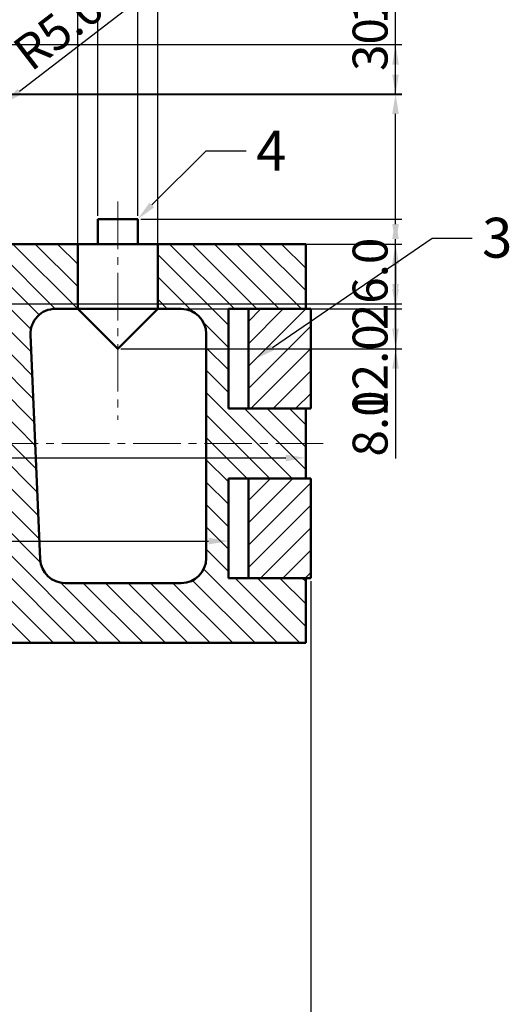
# Model space of a CAD drawing. Units: millimetres. Extents: x -21 to 693, y -570 to 295.
# Tile 5 of 7: x 253 to 352, y -4 to 193. Entities that reach past the tile are written whole.
import ezdxf
from ezdxf import colors
from ezdxf.entities.mleader import LeaderData, LeaderLine
from ezdxf.math import Vec2, Vec3

# ---------------------------------------------------------------- set-up
doc = ezdxf.new("R2010")
doc.units = ezdxf.units.MM
doc.header["$LTSCALE"] = 0.5
doc.linetypes.add('CENTER2', pattern=[28.575, 19.05, -3.175, 3.175, -3.175])
for name, color, linetype, lineweight in [('M-CNTR', 1, 'CENTER2', 18), ('M-DIMS', 2, 'Continuous', 25), ('M-HATC', 8, 'Continuous', 18), ('M-OUTL', 7, 'Continuous', 50), ('M-TEXT', 3, 'Continuous', 25)]:
    doc.layers.add(name, color=color, linetype=linetype, lineweight=lineweight)
doc.styles.get("Standard").update_dxf_attribs({"font": 'arial.ttf'})
doc.dimstyles.new('ISO-25', dxfattribs={"dimtxt": 7, "dimasz": 4, "dimexe": 1.25, "dimexo": 0.625, "dimtad": 1, "dimdec": 0, "dimtxsty": 'Standard', "dimcen": 2.5, "dimadec": 0, "dimazin": 0, "dimtfac": 1, "dimtdec": 0, "dimtofl": 0, "dimtmove": 0, "dimatfit": 3, "dimfxl": 1, "dimarcsym": 0})

# ---------------------------------------------------------------- blocks, each defined once
blk = doc.blocks.new('*U2')
at = {"layer": 'M-CNTR', "color": 0, "transparency": 16777216}
blk.add_line((90.5, 0), (-90.5, 0), dxfattribs=at)
blk = doc.blocks.new('*U4')
at = {"layer": 'M-CNTR', "color": 0, "transparency": 16777216}
blk.add_line((0, 6), (0, -37.73), dxfattribs=at)
blk = doc.blocks.new('*D5')
at = {"layer": 'Defpoints', "color": 0, "ltscale": 0.5, "transparency": 16777216}
for p in [(135.24, 81.11), (311.24, 81.11), (311.24, -8.97)]:
    blk.add_point(p, dxfattribs=at)
at = {"layer": 'M-DIMS', "color": 0, "lineweight": -2, "ltscale": 0.5, "transparency": 16777216}
for p, q in [((135.24, 80.49), (135.24, -10.22)), ((311.24, 80.49), (311.24, -10.22)), ((139.24, -8.97), (307.24, -8.97))]:
    blk.add_line(p, q, dxfattribs=at)
at = {"layer": 'M-DIMS', "color": 0, "ltscale": 0.5, "transparency": 16777216}
for points in [[(139.24, -8.31), (139.24, -9.64), (135.24, -8.97)], [(307.24, -8.31), (307.24, -9.64), (311.24, -8.97)]]:
    blk.add_solid(points, dxfattribs=at)
at = {"layer": 'M-DIMS', "color": 0, "ltscale": 0.5, "transparency": 16777216, "insert": (223.24, -4.58), "char_height": 7, "attachment_point": 5}
blk.add_mtext('%%C175', dxfattribs=at)
blk = doc.blocks.new('*D13')
at = {"layer": 'Defpoints', "color": 0, "ltscale": 0.5, "transparency": 16777216}
for p in [(151.74, 91.11), (294.74, 91.11), (294.74, 88.53)]:
    blk.add_point(p, dxfattribs=at)
at = {"layer": 'M-DIMS', "color": 0, "lineweight": -2, "ltscale": 0.5, "transparency": 16777216}
for p, q in [((151.74, 90.49), (151.74, 87.28)), ((294.74, 90.49), (294.74, 87.28)), ((155.74, 88.53), (290.74, 88.53))]:
    blk.add_line(p, q, dxfattribs=at)
at = {"layer": 'M-DIMS', "color": 0, "ltscale": 0.5, "transparency": 16777216}
for points in [[(155.74, 89.2), (155.74, 87.87), (151.74, 88.53)], [(290.74, 89.2), (290.74, 87.87), (294.74, 88.53)]]:
    blk.add_solid(points, dxfattribs=at)
at = {"layer": 'M-DIMS', "color": 0, "ltscale": 0.5, "transparency": 16777216, "insert": (223.24, 92.93), "char_height": 7, "attachment_point": 5}
blk.add_mtext('%%C158.5', dxfattribs=at)
blk = doc.blocks.new('*D14')
at = {"layer": 'Defpoints', "color": 0, "ltscale": 0.5, "transparency": 16777216}
for p in [(136.24, 108.11), (310.24, 108.11), (310.24, 105.22)]:
    blk.add_point(p, dxfattribs=at)
at = {"layer": 'M-DIMS', "color": 0, "lineweight": -2, "ltscale": 0.5, "transparency": 16777216}
for p, q in [((136.24, 107.49), (136.24, 103.97)), ((310.24, 107.49), (310.24, 103.97)), ((140.24, 105.22), (306.24, 105.22))]:
    blk.add_line(p, q, dxfattribs=at)
at = {"layer": 'M-DIMS', "color": 0, "ltscale": 0.5, "transparency": 16777216}
for points in [[(140.24, 105.89), (140.24, 104.55), (136.24, 105.22)], [(306.24, 105.89), (306.24, 104.55), (310.24, 105.22)]]:
    blk.add_solid(points, dxfattribs=at)
at = {"layer": 'M-DIMS', "color": 0, "ltscale": 0.5, "transparency": 16777216, "insert": (223.24, 109.62), "char_height": 7, "attachment_point": 5}
blk.add_mtext('%%C174', dxfattribs=at)
blk = doc.blocks.new('SCREW-PLUG')
for p, q in [((4, 21), (4, 26)), ((4, 26), (12, 26)), ((12, 26), (12, 21)), ((0, 21), (0, 8)), ((16, 21), (16, 8)), ((0, 8), (8, 0)), ((16, 8), (8, 0))]:
    blk.add_line(p, q)
blk = doc.blocks.new('*D55')
at = {"layer": 'Defpoints', "color": 0, "ltscale": 0.5, "transparency": 16777216}
for p in [(242.24, 148.11), (242.76, 136.11), (328.24, 136.11)]:
    blk.add_point(p, dxfattribs=at)
at = {"layer": 'M-DIMS', "color": 0, "lineweight": -2, "ltscale": 0.5, "transparency": 16777216}
for p, q in [((242.86, 148.11), (329.49, 148.11)), ((328.24, 144.11), (328.24, 140.11)), ((243.39, 136.11), (329.49, 136.11)), ((328.24, 136.11), (328.24, 113.36))]:
    blk.add_line(p, q, dxfattribs=at)
at = {"layer": 'M-DIMS', "color": 0, "ltscale": 0.5, "transparency": 16777216}
for points in [[(327.57, 144.11), (328.9, 144.11), (328.24, 148.11)], [(327.57, 140.11), (328.9, 140.11), (328.24, 136.11)]]:
    blk.add_solid(points, dxfattribs=at)
at = {"layer": 'M-DIMS', "color": 0, "ltscale": 0.5, "transparency": 16777216, "insert": (324.04, 122.74), "char_height": 7, "attachment_point": 5, "rotation": 90}
blk.add_mtext('12.0', dxfattribs=at)
blk = doc.blocks.new('*D57')
at = {"layer": 'Defpoints', "color": 0, "ltscale": 0.5, "transparency": 16777216}
for p in [(280.55, 210.86), (264.55, 135.11), (280.55, 135.11)]:
    blk.add_point(p, dxfattribs=at)
at = {"layer": 'M-DIMS', "color": 0, "lineweight": -2, "ltscale": 0.5, "transparency": 16777216}
for p, q in [((264.55, 135.74), (264.55, 212.11)), ((280.55, 135.74), (280.55, 212.11)), ((268.55, 210.86), (276.55, 210.86)), ((280.55, 210.86), (303.3, 210.86))]:
    blk.add_line(p, q, dxfattribs=at)
at = {"layer": 'M-DIMS', "color": 0, "ltscale": 0.5, "transparency": 16777216}
for points in [[(268.55, 211.53), (268.55, 210.2), (264.55, 210.86)], [(276.55, 211.53), (276.55, 210.2), (280.55, 210.86)]]:
    blk.add_solid(points, dxfattribs=at)
at = {"layer": 'M-DIMS', "color": 0, "ltscale": 0.5, "transparency": 16777216, "insert": (293.93, 215.06), "char_height": 7, "attachment_point": 5}
blk.add_mtext('16.0', dxfattribs=at)
blk = doc.blocks.new('*D58')
at = {"layer": 'Defpoints', "color": 0, "ltscale": 0.5, "transparency": 16777216}
for p in [(276.55, 153.11), (328.24, 153.11), (272.55, 127.11)]:
    blk.add_point(p, dxfattribs=at)
at = {"layer": 'M-DIMS', "color": 0, "lineweight": -2, "ltscale": 0.5, "transparency": 16777216}
for p, q in [((277.18, 153.11), (329.49, 153.11)), ((328.24, 131.11), (328.24, 149.11)), ((273.18, 127.11), (329.49, 127.11))]:
    blk.add_line(p, q, dxfattribs=at)
at = {"layer": 'M-DIMS', "color": 0, "ltscale": 0.5, "transparency": 16777216}
for points in [[(327.57, 149.11), (328.9, 149.11), (328.24, 153.11)], [(327.57, 131.11), (328.9, 131.11), (328.24, 127.11)]]:
    blk.add_solid(points, dxfattribs=at)
at = {"layer": 'M-DIMS', "color": 0, "ltscale": 0.5, "transparency": 16777216, "insert": (324.04, 140.11), "char_height": 7, "attachment_point": 5, "rotation": 90}
blk.add_mtext('26.0', dxfattribs=at)
blk = doc.blocks.new('*D59')
at = {"layer": 'Defpoints', "color": 0, "ltscale": 0.5, "transparency": 16777216}
for p in [(276.55, 210.86), (268.55, 153.11), (276.55, 153.11)]:
    blk.add_point(p, dxfattribs=at)
at = {"layer": 'M-DIMS', "color": 0, "lineweight": -2, "ltscale": 0.5, "transparency": 16777216}
for p, q in [((268.55, 153.74), (268.55, 212.11)), ((276.55, 153.74), (276.55, 212.11)), ((264.55, 210.86), (260.55, 210.86)), ((280.55, 210.86), (298.53, 210.86))]:
    blk.add_line(p, q, dxfattribs=at)
at = {"layer": 'M-DIMS', "color": 0, "ltscale": 0.5, "transparency": 16777216}
for points in [[(264.55, 211.53), (264.55, 210.2), (268.55, 210.86)], [(280.55, 211.53), (280.55, 210.2), (276.55, 210.86)]]:
    blk.add_solid(points, dxfattribs=at)
at = {"layer": 'M-DIMS', "color": 0, "ltscale": 0.5, "transparency": 16777216, "insert": (291.54, 215.06), "char_height": 7, "attachment_point": 5}
blk.add_mtext('8.0', dxfattribs=at)
blk = doc.blocks.new('*D60')
at = {"layer": 'Defpoints', "color": 0, "ltscale": 0.5, "transparency": 16777216}
for p in [(280.55, 135.11), (272.55, 127.11), (328.24, 127.11)]:
    blk.add_point(p, dxfattribs=at)
at = {"layer": 'M-DIMS', "color": 0, "lineweight": -2, "ltscale": 0.5, "transparency": 16777216}
for p, q in [((328.24, 139.11), (328.24, 143.11)), ((281.18, 135.11), (329.49, 135.11)), ((273.18, 127.11), (329.49, 127.11)), ((328.24, 123.11), (328.24, 105.13))]:
    blk.add_line(p, q, dxfattribs=at)
at = {"layer": 'M-DIMS', "color": 0, "ltscale": 0.5, "transparency": 16777216}
for points in [[(327.57, 139.11), (328.9, 139.11), (328.24, 135.11)], [(327.57, 123.11), (328.9, 123.11), (328.24, 127.11)]]:
    blk.add_solid(points, dxfattribs=at)
at = {"layer": 'M-DIMS', "color": 0, "ltscale": 0.5, "transparency": 16777216, "insert": (324.04, 112.12), "char_height": 7, "attachment_point": 5, "rotation": 90}
blk.add_mtext('8.0', dxfattribs=at)
blk = doc.blocks.new('*D62')
at = {"layer": 'Defpoints', "color": 0, "ltscale": 0.5, "transparency": 16777216}
for p in [(245.74, 178.22), (328.24, 178.22), (250.74, 148.11)]:
    blk.add_point(p, dxfattribs=at)
at = {"layer": 'M-DIMS', "color": 0, "lineweight": -2, "ltscale": 0.5, "transparency": 16777216}
for p, q in [((328.24, 178.22), (328.24, 212.58)), ((246.36, 178.22), (329.49, 178.22)), ((328.24, 152.11), (328.24, 174.22)), ((251.36, 148.11), (329.49, 148.11))]:
    blk.add_line(p, q, dxfattribs=at)
at = {"layer": 'M-DIMS', "color": 0, "ltscale": 0.5, "transparency": 16777216}
for points in [[(327.57, 174.22), (328.9, 174.22), (328.24, 178.22)], [(327.57, 152.11), (328.9, 152.11), (328.24, 148.11)]]:
    blk.add_solid(points, dxfattribs=at)
at = {"layer": 'M-DIMS', "color": 0, "ltscale": 0.5, "transparency": 16777216, "insert": (324.04, 197.4), "char_height": 7, "attachment_point": 5, "rotation": 90}
blk.add_mtext('30.105', dxfattribs=at)
blk = doc.blocks.new('*D64')
at = {"layer": 'Defpoints', "color": 0, "ltscale": 0.5, "transparency": 16777216}
for p in [(240.89, 188.11), (328.24, 188.11), (240.89, 178.11)]:
    blk.add_point(p, dxfattribs=at)
at = {"layer": 'M-DIMS', "color": 0, "lineweight": -2, "ltscale": 0.5, "transparency": 16777216}
for p, q in [((328.24, 188.11), (328.24, 210.86)), ((241.51, 188.11), (329.49, 188.11)), ((328.24, 182.11), (328.24, 184.11)), ((241.51, 178.11), (329.49, 178.11))]:
    blk.add_line(p, q, dxfattribs=at)
at = {"layer": 'M-DIMS', "color": 0, "ltscale": 0.5, "transparency": 16777216}
for points in [[(327.57, 184.11), (328.9, 184.11), (328.24, 188.11)], [(327.57, 182.11), (328.9, 182.11), (328.24, 178.11)]]:
    blk.add_solid(points, dxfattribs=at)
at = {"layer": 'M-DIMS', "color": 0, "ltscale": 0.5, "transparency": 16777216, "insert": (324.04, 201.49), "char_height": 7, "attachment_point": 5, "rotation": 90}
blk.add_mtext('10.0', dxfattribs=at)
blk = doc.blocks.new('*D69')
at = {"layer": 'Defpoints', "color": 0, "ltscale": 0.5, "transparency": 16777216}
for p in [(249.7, 176.27), (245.74, 173.22)]:
    blk.add_point(p, dxfattribs=at)
at = {"layer": 'M-DIMS', "color": 0, "lineweight": -2, "ltscale": 0.5, "transparency": 16777216}
for p, q in [((279.98, 199.59), (252.87, 178.71)), ((245.74, 170.72), (245.74, 175.72)), ((243.24, 173.22), (248.24, 173.22))]:
    blk.add_line(p, q, dxfattribs=at)
at = {"layer": 'M-DIMS', "color": 0, "ltscale": 0.5, "transparency": 16777216}
blk.add_solid([(252.46, 179.24), (253.28, 178.18), (249.7, 176.27)], dxfattribs=at)
at = {"layer": 'M-DIMS', "color": 0, "ltscale": 0.5, "transparency": 16777216, "insert": (265.45, 193.7), "char_height": 7, "attachment_point": 5, "rotation": 37.6005}
blk.add_mtext('R5.001', dxfattribs=at)

msp = doc.modelspace()

# ---------------------------------------------------------------- hatches: boundary and pattern name
at = {"layer": 'M-HATC'}
h = msp.add_hatch(dxfattribs=at)
h.set_pattern_fill('ANSI31', color=256, angle=90)
h.paths.add_polyline_path([(136.2368, 148.1134), (136.2368, 135.1134), (151.7368, 135.1134), (151.7368, 115.1134), (136.2368, 115.1134), (136.2368, 108.1134), (156.1864, 108.1134), (156.1864, 130.1134, -0.41421356), (161.1864, 135.1134), (165.9215, 135.1134), (165.9215, 148.1134)])
h.paths.add_polyline_path([(151.7368, 101.1134), (151.7368, 81.1134), (136.2368, 81.1134), (136.2368, 68.1134), (200.7368, 68.1134), (202.4868, 108.1134), (190.4753, 108.1134), (189.4595, 84.8948, -0.40146486), (184.4643, 80.1134), (161.1864, 80.1134, -0.41421356), (156.1864, 85.1134), (156.1864, 108.1134), (136.2368, 108.1134), (136.2368, 101.1134)])
h.paths.add_polyline_path([(204.2368, 148.1134), (195.7368, 148.1134), (181.9215, 148.1134), (181.9215, 135.1134), (186.4331, 135.1134, -0.42707823), (191.4283, 129.8948), (190.4753, 108.1134), (202.4868, 108.1134)])
h.paths.add_polyline_path([(310.2368, 68.1134), (310.2368, 81.1134), (294.7368, 81.1134), (294.7368, 101.1134), (310.2368, 101.1134), (310.2368, 108.1134), (290.2872, 108.1134), (290.2872, 85.1134, -0.41421356), (285.2872, 80.1134), (262.0093, 80.1134, -0.40146486), (257.0141, 84.8948), (255.9983, 108.1134), (243.9868, 108.1134), (245.7368, 68.1134)])
h.paths.add_polyline_path([(243.9868, 108.1134), (255.9983, 108.1134), (255.0454, 129.8948, -0.42707823), (260.0406, 135.1134), (264.5522, 135.1134), (264.5522, 148.1134), (242.2368, 148.1134)])
h.paths.add_polyline_path([(280.5522, 135.1134), (285.2872, 135.1134, -0.41421356), (290.2872, 130.1134), (290.2872, 108.1134), (310.2368, 108.1134), (310.2368, 115.1134), (294.7368, 115.1134), (294.7368, 135.1134), (310.2368, 135.1134), (310.2368, 148.1134), (280.5522, 148.1134)])
h = msp.add_hatch(dxfattribs=at)
h.set_pattern_fill('ANSI31', color=256)
h.paths.add_polyline_path([(311.2368, 135.1134), (298.7368, 135.1134), (298.7368, 115.1134), (311.2368, 115.1134)])
h.paths.add_polyline_path([(298.7368, 101.1134), (298.7368, 81.1134), (311.2368, 81.1134), (311.2368, 101.1134)])

# ---------------------------------------------------------------- linework, layer by layer
at = {"layer": 'M-OUTL'}
for p, q in [((310.2368, 148.1134), (136.2368, 148.1134)), ((310.2368, 148.1134), (310.2368, 135.1134)), ((285.2872, 135.1134), (260.0406, 135.1134)), ((294.7368, 115.1134), (294.7368, 135.1134)), ((294.7368, 135.1134), (311.2368, 135.1134)), ((298.7368, 115.1134), (298.7368, 135.1134)), ((311.2368, 135.1134), (311.2368, 115.1134)), ((257.0141, 84.8948), (255.0454, 129.8948)), ((290.2872, 130.1134), (290.2872, 85.1134)), ((311.2368, 115.1134), (294.7368, 115.1134)), ((310.2368, 101.1134), (310.2368, 115.1134)), ((294.7368, 81.1134), (294.7368, 101.1134)), ((294.7368, 101.1134), (311.2368, 101.1134)), ((298.7368, 81.1134), (298.7368, 101.1134)), ((311.2368, 101.1134), (311.2368, 81.1134)), ((311.2368, 81.1134), (294.7368, 81.1134)), ((310.2368, 68.1134), (310.2368, 81.1134)), ((285.2872, 80.1134), (262.0093, 80.1134)), ((136.2368, 68.1134), (310.2368, 68.1134))]:
    msp.add_line(p, q, dxfattribs=at)
for centre, start, end in [((260.0406, 130.1134), 90, 182.505093), ((285.2872, 130.1134), 360, 90), ((285.2872, 85.1134), 270, 360), ((262.0093, 85.1134), 182.505093, 270)]:
    msp.add_arc(centre, 5, start, end, dxfattribs=at)

# ---------------------------------------------------------------- block references
at = {"layer": 'M-CNTR'}
for name, p in [('*U4', (272.5522, 150.6134)), ('*U2', (223.2368, 108.1134))]:
    msp.add_blockref(name, p, dxfattribs=at)
at = {"layer": 'M-OUTL'}
msp.add_blockref('SCREW-PLUG', (264.5526, 127.113), dxfattribs=at)

# ---------------------------------------------------------------- dimensions: what is measured, and where the dimension line sits
at = {"layer": 'M-DIMS', "ltscale": 0.5}
for base, p1, p2, picture, middle in [((276.5522, 210.864), (268.5522, 153.1134), (276.5522, 153.1134), '*D59', (291.5421, 215.063)), ((280.5522, 210.864), (264.5522, 135.1134), (280.5522, 135.1134), '*D57', (293.9272, 215.063))]:
    dim = msp.add_linear_dim(base=base, p1=p1, p2=p2, dimstyle='ISO-25', override={"dimdec": 1, "dimlfac": 1, "dimrnd": 0, "dimzin": 0, "dimdsep": 46, "dimlunit": 2}, dxfattribs=at)
    dim.commit()
    dim.dimension.update_dxf_attribs({"geometry": picture, "text_midpoint": middle})
for base, p1, p2, override, picture, middle in [((328.23683, 178.21793), (250.73683, 148.11336), (245.73683, 178.21793), {"dimdec": 3, "dimlfac": 1, "dimrnd": 0, "dimzin": 0, "dimdsep": 46, "dimlunit": 2}, '*D62', (324.03543, 197.39682)), ((328.2368, 188.1134), (240.8872, 178.1134), (240.8872, 188.1134), {"dimdec": 1, "dimlfac": 1, "dimrnd": 0, "dimzin": 0, "dimdsep": 46, "dimlunit": 2}, '*D64', (324.0378, 201.4884)), ((328.2368, 153.1134), (272.5522, 127.1134), (276.5522, 153.1134), {"dimdec": 1, "dimlfac": 1, "dimrnd": 0, "dimzin": 0, "dimdsep": 46, "dimlunit": 2}, '*D58', (324.0378, 140.1134)), ((328.2368, 136.1134), (242.2368, 148.1134), (242.7618, 136.1134), {"dimdec": 1, "dimlfac": 1, "dimrnd": 0, "dimzin": 0, "dimdsep": 46, "dimlunit": 2}, '*D55', (324.0378, 122.7384)), ((328.2368, 127.1134), (280.5522, 135.1134), (272.5522, 127.1134), {"dimdec": 1, "dimlfac": 1, "dimrnd": 0, "dimzin": 0, "dimdsep": 46, "dimlunit": 2}, '*D60', (324.0378, 112.1234))]:
    dim = msp.add_linear_dim(base=base, p1=p1, p2=p2, angle=90, dimstyle='ISO-25', override=override, dxfattribs=at)
    dim.commit()
    dim.dimension.update_dxf_attribs({"geometry": picture, "text_midpoint": middle})
dim = msp.add_radius_dim(center=(245.7368, 173.2169), mpoint=(249.6991, 176.2683), dimstyle='ISO-25', override={"dimdec": 3, "dimlfac": 1, "dimrnd": 0, "dimzin": 0, "dimdsep": 46, "dimlunit": 2}, dxfattribs=at)
dim.commit()
dim.dimension.update_dxf_attribs({"geometry": '*D69', "text_midpoint": (265.4465, 193.6955)})
for base, p1, p2, text, picture, middle in [((310.2368, 105.2205), (136.2368, 108.1134), (310.2368, 108.1134), '%%C<>', '*D14', (223.2368, 109.6152)), ((294.7368, 88.5333), (151.7368, 91.1134), (294.7368, 91.1134), '%%C158.5', '*D13', (223.2368, 92.9281))]:
    dim = msp.add_linear_dim(base=base, p1=p1, p2=p2, text=text, dimstyle='ISO-25', override={"dimclrd": 0, "dimclre": 0, "dimclrt": 0}, dxfattribs=at)
    dim.commit()
    dim.dimension.update_dxf_attribs({"geometry": picture, "text_midpoint": middle})
dim = msp.add_linear_dim(base=(311.2368, -8.9735), p1=(135.2368, 81.1134), p2=(311.2368, 81.1134), text='%%C175', dimstyle='ISO-25', override={"dimclrd": 0, "dimclre": 0, "dimclrt": 0}, dxfattribs=at)
dim.commit()
dim.dimension.update_dxf_attribs({"geometry": '*D5', "text_midpoint": (223.2368, -8.9735), "dimtype": 160})

# ---------------------------------------------------------------- leaders
at = {"layer": 'M-TEXT', "ltscale": 0.5}
ml = msp.add_multileader_mtext('Standard', dxfattribs=at)
ml.set_content('4', color=256)
ml.set_leader_properties()
ml.build(insert=Vec2(0, 0))
ctx = ml.context
ctx.base_point, ctx.char_height, ctx.plane_origin = Vec3(298.2766, 166.8379), 8, Vec3(276.5522, 153.1134)
notes = []
notes.append((ctx, [(0, (1, 1, 0), (290.2766, 166.8379), (1, 0), 8, [(0, [(276.5522, 153.1134)], 0, [])])]))
ctx.mtext.insert, ctx.mtext.flow_direction = Vec3(300.2766, 170.8379), 5
ml = msp.add_multileader_mtext('Standard', dxfattribs=at)
ml.set_content('3', color=256)
ml.set_leader_properties()
ml.build(insert=Vec2(0, 0))
ctx = ml.context
ctx.base_point, ctx.char_height, ctx.plane_origin = Vec3(343.5836, 149.3072), 8, Vec3(300.2368, 125.1134)
notes.append((ctx, [(0, (1, 1, 0), (335.5836, 149.3072), (1, 0), 8, [(0, [(300.2368, 125.1134)], 0, [])])]))
ctx.mtext.insert, ctx.mtext.flow_direction = Vec3(345.5836, 153.3782), 5
for ctx, leaders in notes:
    for number, flags, end, landing, length, lines in leaders:
        leader = LeaderData()
        leader.index, (leader.has_last_leader_line, leader.has_dogleg_vector, leader.attachment_direction) = number, flags
        leader.last_leader_point, leader.dogleg_vector, leader.dogleg_length = Vec3(end), Vec3(landing), length
        for number, points, colour, breaks in lines:
            line = LeaderLine()
            line.index, line.vertices, line.color, line.breaks = number, Vec3.list(points), colors.encode_raw_color(colour), breaks
            leader.lines.append(line)
        ctx.leaders.append(leader)

doc.saveas('drawing.dxf')
